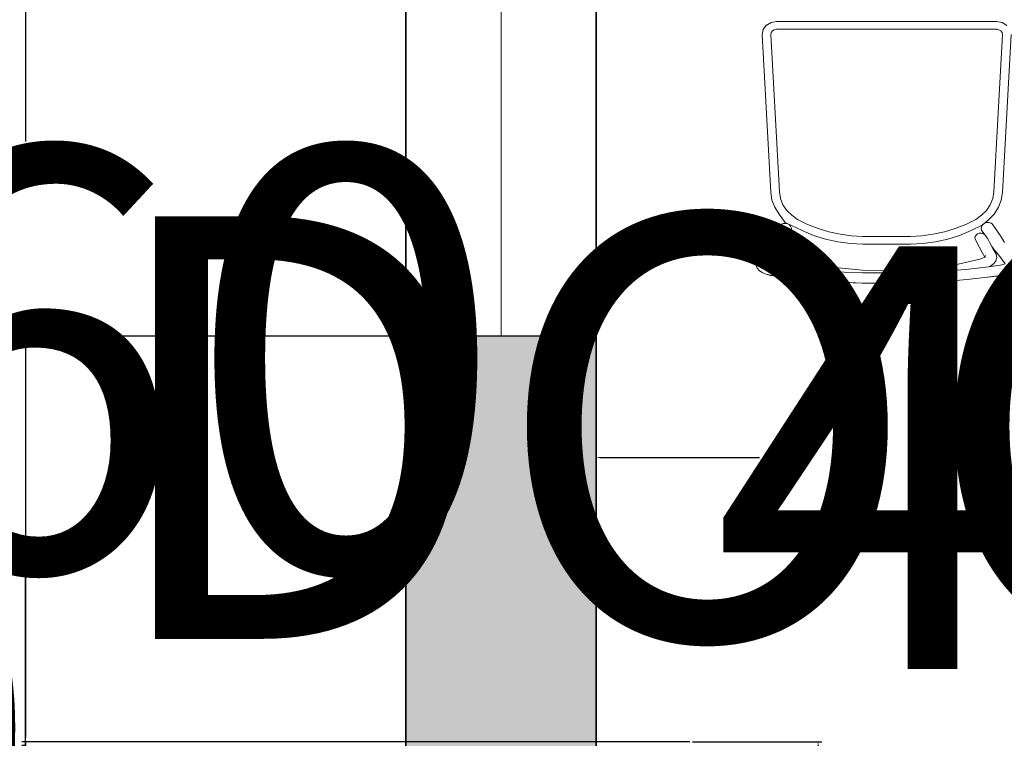
# Model space of a CAD drawing. Units: inches. Extents: x 305 to 776, y 38 to 479.
# Tile 5 of 14: x 372 to 419, y 231 to 265. Entities that reach past the tile are written whole.
import ezdxf

# ---------------------------------------------------------------- set-up
doc = ezdxf.new("R2010")
doc.units = ezdxf.units.IN
doc.header["$MEASUREMENT"] = 0
for name, color, linetype, lineweight in [('A-ANNO-DIMS', 2, 'Continuous', 18), ('A-FURN', 8, 'Continuous', 18), ('A-GLAZ', 4, 'Continuous', 20), ('A-WALL', 7, 'Continuous', 35), ('A-WALL-PATT', 252, 'Continuous', 13)]:
    doc.layers.add(name, color=color, linetype=linetype, lineweight=lineweight)
doc.styles.get("Standard").update_dxf_attribs({"font": 'arial.ttf'})
doc.dimstyles.get("Standard").update_dxf_attribs({"dimtxt": 20, "dimasz": 0.18, "dimexe": 0.18, "dimexo": 0.0625, "dimgap": 0.09, "dimtad": 0, "dimtih": 1, "dimtoh": 1, "dimdec": 4, "dimzin": 0, "dimdsep": 46, "dimtxsty": 'Standard', "dimcen": 0.09, "dimadec": 0, "dimazin": 0, "dimtfac": 1, "dimtdec": 4, "dimtofl": 0, "dimtmove": 0, "dimatfit": 3, "dimfxl": 1, "dimtolj": 1, "dimtzin": 0, "dimarcsym": 0})

# ---------------------------------------------------------------- blocks, each defined once
blk = doc.blocks.new('W3')
blk.add_line((906.212, 308.312), (886.612, 308.312))
blk.add_lwpolyline([(886.612, 303.812), (906.212, 303.812), (906.212, 312.812), (886.612, 312.812)])
blk = doc.blocks.new('D')
for p, q in [((1074.026, 474.114), (1073.821, 473.841)), ((1074.026, 474.113), (1073.821, 473.84)), ((1074.333, 474.296), (1074.026, 474.114)), ((1074.333, 474.295), (1074.026, 474.113)), ((1074.695, 474.36), (1074.333, 474.296)), ((1074.695, 474.359), (1074.333, 474.295)), ((1089.074, 474.36), (1074.695, 474.36)), ((1089.074, 474.359), (1074.695, 474.359)), ((1089.436, 474.296), (1089.074, 474.36)), ((1089.436, 474.295), (1089.074, 474.359)), ((1089.743, 474.114), (1089.436, 474.296)), ((1089.743, 474.113), (1089.436, 474.295)), ((1073.821, 473.841), (1073.749, 473.519)), ((1073.821, 473.84), (1073.749, 473.518)), ((1073.749, 473.519), (1074.316, 463.208)), ((1073.749, 473.518), (1074.316, 463.207)), ((1074.316, 473.518), (1074.345, 473.647)), ((1074.883, 463.232), (1074.316, 473.518)), ((1074.345, 473.647), (1074.427, 473.756)), ((1074.427, 473.756), (1074.55, 473.829)), ((1074.55, 473.829), (1074.695, 473.855)), ((1074.695, 473.855), (1089.074, 473.855)), ((1089.453, 473.518), (1088.886, 463.232)), ((1089.074, 473.855), (1089.219, 473.829)), ((1089.219, 473.829), (1089.342, 473.756)), ((1089.342, 473.756), (1089.424, 473.647)), ((1089.424, 473.647), (1089.453, 473.518)), ((1089.453, 463.208), (1090.02, 473.519)), ((1089.453, 463.207), (1090.02, 473.518)), ((1074.316, 463.208), (1074.397, 462.709)), ((1074.316, 463.207), (1074.397, 462.708)), ((1074.954, 462.807), (1074.883, 463.232)), ((1088.886, 463.232), (1088.815, 462.807)), ((1089.372, 462.709), (1089.453, 463.208)), ((1089.372, 462.708), (1089.453, 463.207)), ((1074.397, 462.709), (1074.58, 462.232)), ((1074.397, 462.708), (1074.58, 462.231)), ((1075.116, 462.403), (1074.954, 462.807)), ((1075.363, 462.034), (1075.116, 462.403)), ((1088.653, 462.403), (1088.406, 462.034)), ((1088.815, 462.807), (1088.653, 462.403)), ((1089.189, 462.232), (1089.372, 462.709)), ((1089.189, 462.231), (1089.372, 462.708)), ((1074.58, 462.232), (1074.859, 461.794)), ((1074.58, 462.231), (1074.859, 461.793)), ((1074.859, 461.794), (1075.262, 461.238)), ((1074.859, 461.793), (1075.262, 461.238)), ((1075.686, 461.714), (1075.363, 462.034)), ((1076.065, 461.447), (1075.686, 461.714)), ((1088.083, 461.714), (1087.704, 461.447)), ((1088.406, 462.034), (1088.083, 461.714)), ((1088.545, 461.409), (1088.91, 461.794)), ((1088.545, 461.408), (1088.91, 461.793)), ((1088.91, 461.794), (1089.189, 462.232)), ((1088.91, 461.793), (1089.189, 462.231)), ((1074.941, 461.071), (1074.459, 460.363)), ((1074.941, 461.071), (1074.459, 460.363)), ((1075.068, 461.151), (1074.941, 461.071)), ((1074.994, 461.113), (1074.941, 461.071)), ((1075.053, 461.145), (1074.994, 461.113)), ((1075.118, 461.169), (1075.053, 461.145)), ((1075.22, 461.186), (1075.068, 461.151)), ((1075.186, 461.183), (1075.118, 461.169)), ((1075.256, 461.187), (1075.186, 461.183)), ((1075.375, 461.17), (1075.22, 461.186)), ((1075.326, 461.181), (1075.256, 461.187)), ((1075.262, 461.238), (1075.339, 461.202)), ((1076.372, 460.712), (1075.262, 461.238)), ((1075.339, 461.202), (1075.326, 461.181)), ((1075.513, 461.105), (1075.375, 461.17)), ((1075.616, 461.001), (1075.513, 461.105)), ((1075.67, 460.87), (1075.616, 461.001)), ((1076.72, 461.12), (1076.065, 461.447)), ((1077.406, 460.848), (1076.72, 461.12)), ((1087.049, 461.12), (1086.363, 460.848)), ((1087.704, 461.447), (1087.049, 461.12)), ((1087.397, 460.712), (1088.111, 461.071)), ((1088.098, 461.017), (1088.06, 460.879)), ((1088.189, 461.132), (1088.098, 461.017)), ((1088.111, 461.071), (1088.545, 461.408)), ((1088.321, 461.212), (1088.189, 461.132)), ((1088.475, 461.243), (1088.321, 461.212)), ((1088.362, 461.267), (1088.545, 461.409)), ((1088.392, 461.234), (1088.362, 461.267)), ((1088.472, 461.244), (1088.392, 461.234)), ((1088.552, 461.241), (1088.472, 461.244)), ((1088.633, 461.224), (1088.475, 461.243)), ((1088.631, 461.225), (1088.552, 461.241)), ((1088.705, 461.196), (1088.631, 461.225)), ((1088.772, 461.155), (1088.633, 461.224)), ((1088.772, 461.156), (1088.705, 461.196)), ((1089.31, 460.363), (1088.772, 461.156)), ((1088.772, 461.155), (1089.31, 460.363)), ((1074.459, 460.363), (1074.192, 459.938)), ((1074.459, 460.363), (1074.192, 459.937)), ((1075.308, 460.2), (1075.415, 460.372)), ((1075.489, 460.462), (1075.415, 460.372)), ((1075.448, 460.42), (1075.61, 460.603)), ((1075.593, 460.525), (1075.489, 460.462)), ((1075.714, 460.554), (1075.593, 460.525)), ((1075.61, 460.603), (1075.668, 460.732)), ((1075.668, 460.732), (1075.67, 460.87)), ((1075.839, 460.545), (1075.714, 460.554)), ((1075.954, 460.5), (1075.839, 460.545)), ((1076.045, 460.423), (1075.954, 460.5)), ((1076.102, 460.324), (1076.045, 460.423)), ((1076.372, 460.712), (1077.118, 460.398)), ((1077.118, 460.398), (1077.895, 460.15)), ((1078.116, 460.631), (1077.406, 460.848)), ((1078.845, 460.472), (1078.116, 460.631)), ((1079.588, 460.372), (1078.845, 460.472)), ((1080.337, 460.332), (1079.588, 460.372)), ((1084.181, 460.372), (1083.432, 460.332)), ((1084.924, 460.472), (1084.181, 460.372)), ((1085.653, 460.631), (1084.924, 460.472)), ((1086.363, 460.848), (1085.653, 460.631)), ((1085.874, 460.15), (1086.651, 460.398)), ((1086.651, 460.398), (1087.397, 460.712)), ((1087.724, 460.423), (1087.667, 460.324)), ((1087.815, 460.5), (1087.724, 460.423)), ((1087.93, 460.545), (1087.815, 460.5)), ((1088.055, 460.554), (1087.93, 460.545)), ((1088.176, 460.525), (1088.055, 460.554)), ((1088.06, 460.879), (1088.08, 460.739)), ((1088.08, 460.739), (1088.155, 460.615)), ((1088.321, 460.42), (1088.155, 460.615)), ((1088.28, 460.462), (1088.176, 460.525)), ((1088.354, 460.372), (1088.28, 460.462)), ((1088.461, 460.2), (1088.354, 460.372)), ((1089.577, 459.938), (1089.31, 460.363)), ((1089.31, 460.363), (1089.577, 459.937)), ((1074.192, 459.938), (1073.839, 459.39)), ((1074.192, 459.937), (1073.839, 459.39)), ((1075.147, 459.905), (1074.97, 459.586)), ((1075.288, 460.169), (1075.147, 459.905)), ((1075.308, 460.2), (1075.288, 460.169)), ((1075.976, 459.888), (1075.827, 459.611)), ((1076.119, 460.213), (1075.976, 459.888)), ((1076.119, 460.213), (1076.102, 460.324)), ((1077.895, 460.15), (1078.696, 459.971)), ((1078.696, 459.971), (1079.513, 459.863)), ((1079.513, 459.863), (1080.337, 459.827)), ((1083.432, 460.332), (1080.337, 460.332)), ((1080.337, 459.827), (1083.432, 459.827)), ((1083.432, 459.827), (1084.256, 459.863)), ((1084.256, 459.863), (1085.073, 459.971)), ((1085.073, 459.971), (1085.874, 460.15)), ((1087.667, 460.324), (1087.65, 460.213)), ((1087.65, 460.213), (1087.793, 459.888)), ((1087.793, 459.888), (1087.942, 459.611)), ((1088.461, 460.2), (1088.481, 460.169)), ((1088.481, 460.169), (1088.622, 459.905)), ((1088.622, 459.905), (1088.799, 459.586)), ((1073.839, 459.39), (1073.441, 458.781)), ((1073.839, 459.39), (1073.441, 458.78)), ((1074.899, 459.526), (1074.503, 459.012)), ((1074.735, 459.167), (1074.693, 458.942)), ((1074.97, 459.586), (1074.735, 459.167)), ((1075.019, 459.675), (1074.899, 459.526)), ((1075.419, 459.083), (1075.441, 459.015)), ((1075.646, 459.285), (1075.472, 458.985)), ((1075.827, 459.611), (1075.646, 459.285)), ((1087.942, 459.611), (1088.123, 459.285)), ((1088.123, 459.285), (1088.297, 458.985)), ((1088.35, 459.083), (1088.328, 459.015)), ((1088.75, 459.675), (1088.87, 459.526)), ((1088.799, 459.586), (1089.034, 459.167)), ((1088.87, 459.526), (1089.265, 459.012)), ((1089.034, 459.167), (1089.076, 458.942)), ((1073.369, 458.627), (1073.341, 458.506)), ((1073.341, 458.506), (1073.369, 458.626)), ((1073.341, 458.506), (1073.38, 458.366)), ((1073.341, 458.506), (1073.38, 458.365)), ((1073.402, 458.733), (1073.369, 458.627)), ((1073.402, 458.732), (1073.369, 458.626)), ((1073.441, 458.781), (1073.402, 458.733)), ((1073.402, 458.732), (1073.441, 458.78)), ((1073.99, 458.675), (1074.082, 458.587)), ((1074.082, 458.587), (1074.149, 458.547)), ((1074.149, 458.547), (1074.284, 458.496)), ((1074.503, 459.012), (1074.155, 458.545)), ((1074.284, 458.496), (1074.454, 458.449)), ((1074.454, 458.449), (1075.569, 458.308)), ((1074.727, 458.826), (1074.693, 458.942)), ((1074.727, 458.826), (1074.764, 458.711)), ((1074.764, 458.711), (1074.907, 458.531)), ((1074.907, 458.531), (1075.103, 458.387)), ((1075.441, 459.015), (1075.456, 458.996)), ((1075.456, 458.996), (1075.511, 458.956)), ((1075.511, 458.956), (1075.628, 458.905)), ((1075.628, 458.905), (1075.79, 458.847)), ((1075.79, 458.847), (1077.219, 458.522)), ((1077.219, 458.522), (1078.734, 458.273)), ((1086.55, 458.522), (1085.035, 458.273)), ((1087.979, 458.847), (1086.55, 458.522)), ((1088.141, 458.905), (1087.979, 458.847)), ((1088.258, 458.956), (1088.141, 458.905)), ((1089.315, 458.449), (1088.2, 458.308)), ((1088.313, 458.996), (1088.258, 458.956)), ((1088.328, 459.015), (1088.313, 458.996)), ((1088.862, 458.531), (1088.666, 458.387)), ((1089.005, 458.711), (1088.862, 458.531)), ((1089.042, 458.826), (1089.005, 458.711)), ((1089.042, 458.826), (1089.076, 458.942)), ((1089.265, 459.012), (1089.614, 458.545)), ((1089.485, 458.496), (1089.315, 458.449)), ((1089.62, 458.547), (1089.485, 458.496)), ((1073.38, 458.366), (1073.421, 458.251)), ((1073.421, 458.25), (1073.38, 458.365)), ((1073.421, 458.251), (1073.589, 458.075)), ((1073.421, 458.25), (1073.589, 458.074)), ((1073.589, 458.075), (1073.794, 457.953)), ((1073.589, 458.074), (1073.794, 457.952)), ((1073.794, 457.953), (1074.023, 457.865)), ((1073.794, 457.952), (1074.023, 457.864)), ((1074.023, 457.865), (1074.289, 457.791)), ((1074.023, 457.864), (1074.289, 457.79)), ((1074.289, 457.791), (1075.47, 457.642)), ((1074.289, 457.79), (1075.47, 457.641)), ((1075.103, 458.387), (1075.165, 458.359)), ((1075.569, 458.308), (1076.732, 458.181)), ((1076.732, 458.181), (1077.91, 458.079)), ((1077.91, 458.079), (1079.101, 458.005)), ((1078.734, 458.273), (1080.296, 458.126)), ((1079.101, 458.005), (1080.302, 457.96)), ((1080.296, 458.126), (1081.884, 458.091)), ((1080.302, 457.96), (1081.509, 457.945)), ((1082.26, 457.945), (1081.509, 457.945)), ((1083.473, 458.126), (1081.884, 458.091)), ((1083.467, 457.96), (1082.26, 457.945)), ((1084.668, 458.005), (1083.467, 457.96)), ((1085.035, 458.273), (1083.473, 458.126)), ((1085.859, 458.079), (1084.668, 458.005)), ((1087.037, 458.181), (1085.859, 458.079)), ((1088.2, 458.308), (1087.037, 458.181)), ((1088.299, 457.642), (1089.48, 457.791)), ((1089.48, 457.79), (1088.299, 457.641)), ((1088.666, 458.387), (1088.604, 458.359)), ((1089.48, 457.791), (1089.746, 457.865)), ((1089.746, 457.864), (1089.48, 457.79)), ((1075.47, 457.642), (1076.649, 457.513)), ((1075.47, 457.641), (1076.649, 457.512)), ((1076.649, 457.513), (1077.847, 457.409)), ((1076.649, 457.512), (1077.847, 457.409)), ((1077.847, 457.409), (1079.059, 457.334)), ((1077.847, 457.409), (1079.059, 457.333)), ((1079.059, 457.334), (1080.28, 457.288)), ((1079.059, 457.333), (1080.28, 457.287)), ((1080.28, 457.288), (1081.503, 457.273)), ((1080.28, 457.287), (1081.503, 457.272)), ((1081.503, 457.273), (1082.266, 457.273)), ((1082.266, 457.272), (1081.503, 457.272)), ((1082.266, 457.273), (1083.489, 457.288)), ((1083.489, 457.287), (1082.266, 457.272)), ((1083.489, 457.288), (1084.71, 457.334)), ((1084.71, 457.333), (1083.489, 457.287)), ((1084.71, 457.334), (1085.922, 457.409)), ((1085.922, 457.409), (1084.71, 457.333)), ((1085.922, 457.409), (1087.12, 457.513)), ((1087.12, 457.512), (1085.922, 457.409)), ((1087.12, 457.513), (1088.299, 457.642)), ((1088.299, 457.641), (1087.12, 457.512))]:
    blk.add_line(p, q)
blk = doc.blocks.new('*D19')
at = {"layer": 'A-ANNO-DIMS', "color": 0, "lineweight": -2, "transparency": 16777216}
for p, q in [((557.633, 250.82), (557.633, 245.977)), ((589.133, 250.82), (589.133, 245.977)), ((557.633, 246.157), (557.453, 246.157)), ((588.953, 246.157), (557.813, 246.157))]:
    blk.add_line(p, q, dxfattribs=at)
at = {"layer": 'A-ANNO-DIMS', "color": 0, "transparency": 16777216}
for points in [[(557.813, 246.187), (557.813, 246.127), (557.633, 246.157)], [(588.953, 246.187), (588.953, 246.127), (589.133, 246.157)]]:
    blk.add_solid(points, dxfattribs=at)
at = {"layer": 'Defpoints', "color": 0, "transparency": 16777216}
for p in [(557.633, 250.882), (589.133, 250.882), (557.633, 246.157)]:
    blk.add_point(p, dxfattribs=at)
at = {"layer": 'A-ANNO-DIMS', "color": 0, "transparency": 16777216, "insert": (463.393, 246.157), "char_height": 20, "attachment_point": 5}
blk.add_mtext('\\A1;DOOR 32 TYP.', dxfattribs=at)
blk = doc.blocks.new('*D33')
at = {"layer": 'A-ANNO-DIMS', "color": 0, "lineweight": -2, "transparency": 16777216}
for p, q in [((440.927, 307.949), (449.29, 307.949)), ((449.11, 307.769), (449.11, 290.896)), ((449.11, 253.161), (449.11, 270.034)), ((440.927, 252.981), (449.29, 252.981))]:
    blk.add_line(p, q, dxfattribs=at)
at = {"layer": 'A-ANNO-DIMS', "color": 0, "transparency": 16777216}
for points in [[(449.08, 307.769), (449.14, 307.769), (449.11, 307.949)], [(449.08, 253.161), (449.14, 253.161), (449.11, 252.981)]]:
    blk.add_solid(points, dxfattribs=at)
at = {"layer": 'Defpoints', "color": 0, "transparency": 16777216}
for p in [(440.864, 307.949), (449.11, 307.949), (440.864, 252.981)]:
    blk.add_point(p, dxfattribs=at)
at = {"layer": 'A-ANNO-DIMS', "color": 0, "transparency": 16777216, "insert": (449.11, 280.465), "char_height": 20, "attachment_point": 5}
blk.add_mtext('\\A1;DINING SET 55', dxfattribs=at)
blk = doc.blocks.new('*D34')
at = {"layer": 'A-ANNO-DIMS', "color": 0, "lineweight": -2, "transparency": 16777216}
for p, q in [((399.621, 252.919), (399.621, 244.556)), ((440.864, 252.919), (440.864, 244.556)), ((399.801, 244.736), (407.356, 244.736)), ((440.684, 244.736), (433.129, 244.736))]:
    blk.add_line(p, q, dxfattribs=at)
at = {"layer": 'A-ANNO-DIMS', "color": 0, "transparency": 16777216}
for points in [[(399.801, 244.766), (399.801, 244.706), (399.621, 244.736)], [(440.684, 244.766), (440.684, 244.706), (440.864, 244.736)]]:
    blk.add_solid(points, dxfattribs=at)
at = {"layer": 'Defpoints', "color": 0, "transparency": 16777216}
for p in [(399.621, 252.981), (440.864, 252.981), (440.864, 244.736)]:
    blk.add_point(p, dxfattribs=at)
at = {"layer": 'A-ANNO-DIMS', "color": 0, "transparency": 16777216, "insert": (420.242, 244.736), "char_height": 20, "attachment_point": 5}
blk.add_mtext('\\A1;41', dxfattribs=at)
blk = doc.blocks.new('*D37')
at = {"layer": 'A-ANNO-DIMS', "color": 0, "lineweight": -2, "transparency": 16777216}
for p, q in [((476.346, 237.029), (483.222, 237.029)), ((483.042, 236.849), (483.042, 224.939)), ((483.042, 192.153), (483.042, 204.063)), ((476.346, 191.973), (483.222, 191.973))]:
    blk.add_line(p, q, dxfattribs=at)
at = {"layer": 'A-ANNO-DIMS', "color": 0, "transparency": 16777216}
for points in [[(483.012, 236.849), (483.072, 236.849), (483.042, 237.029)], [(483.012, 192.153), (483.072, 192.153), (483.042, 191.973)]]:
    blk.add_solid(points, dxfattribs=at)
at = {"layer": 'Defpoints', "color": 0, "transparency": 16777216}
for p in [(476.283, 237.029), (483.042, 237.029), (476.283, 191.973)]:
    blk.add_point(p, dxfattribs=at)
at = {"layer": 'A-ANNO-DIMS', "color": 0, "transparency": 16777216, "insert": (483.042, 214.501), "char_height": 20, "attachment_point": 5}
blk.add_mtext('\\A1;COFFEE TABLE 45', dxfattribs=at)
blk = doc.blocks.new('*D39')
at = {"layer": 'A-ANNO-DIMS', "color": 0, "lineweight": -2, "transparency": 16777216}
for p, q in [((404.195, 231.292), (410.313, 231.292)), ((410.133, 231.112), (410.133, 221.593)), ((410.133, 191.472), (410.133, 200.99)), ((404.195, 191.292), (410.313, 191.292))]:
    blk.add_line(p, q, dxfattribs=at)
at = {"layer": 'A-ANNO-DIMS', "color": 0, "transparency": 16777216}
for points in [[(410.103, 231.112), (410.163, 231.112), (410.133, 231.292)], [(410.103, 191.472), (410.163, 191.472), (410.133, 191.292)]]:
    blk.add_solid(points, dxfattribs=at)
at = {"layer": 'Defpoints', "color": 0, "transparency": 16777216}
for p in [(404.133, 231.292), (410.133, 231.292), (404.133, 191.292)]:
    blk.add_point(p, dxfattribs=at)
at = {"layer": 'A-ANNO-DIMS', "color": 0, "transparency": 16777216, "insert": (410.133, 211.292), "char_height": 20, "attachment_point": 5}
blk.add_mtext('\\A1;TV 40', dxfattribs=at)
blk = doc.blocks.new('*D46')
at = {"layer": 'A-ANNO-DIMS', "color": 0, "lineweight": -2, "transparency": 16777216}
for p, q in [((390.57, 429.382), (372.451, 429.382)), ((372.631, 429.202), (372.631, 259.69)), ((372.631, 69.562), (372.631, 239.074)), ((390.57, 69.382), (372.451, 69.382))]:
    blk.add_line(p, q, dxfattribs=at)
at = {"layer": 'A-ANNO-DIMS', "color": 0, "transparency": 16777216}
for points in [[(372.601, 429.202), (372.661, 429.202), (372.631, 429.382)], [(372.601, 69.562), (372.661, 69.562), (372.631, 69.382)]]:
    blk.add_solid(points, dxfattribs=at)
at = {"layer": 'Defpoints', "color": 0, "transparency": 16777216}
for p in [(372.631, 429.382), (390.633, 429.382), (390.633, 69.382)]:
    blk.add_point(p, dxfattribs=at)
at = {"layer": 'A-ANNO-DIMS', "color": 0, "transparency": 16777216, "insert": (372.631, 249.382), "char_height": 20, "attachment_point": 5}
blk.add_mtext('\\A1;360', dxfattribs=at)
blk = doc.blocks.new('*D62')
at = {"layer": 'A-ANNO-DIMS', "color": 0, "lineweight": -2, "transparency": 16777216}
for p, q in [((399.633, 336.32), (399.633, 51.201)), ((423.233, 336.32), (423.233, 51.201)), ((399.813, 51.381), (423.053, 51.381)), ((423.233, 51.381), (423.413, 51.381))]:
    blk.add_line(p, q, dxfattribs=at)
at = {"layer": 'A-ANNO-DIMS', "color": 0, "transparency": 16777216}
for points in [[(399.813, 51.411), (399.813, 51.351), (399.633, 51.381)], [(423.053, 51.411), (423.053, 51.351), (423.233, 51.381)]]:
    blk.add_solid(points, dxfattribs=at)
at = {"layer": 'Defpoints', "color": 0, "transparency": 16777216}
for p in [(399.633, 336.382), (423.233, 336.382), (423.233, 51.381)]:
    blk.add_point(p, dxfattribs=at)
at = {"layer": 'A-ANNO-DIMS', "color": 0, "transparency": 16777216, "insert": (449.642, 51.381), "char_height": 20, "attachment_point": 5}
blk.add_mtext('\\A1;23.6', dxfattribs=at)
blk = doc.blocks.new('*D65')
at = {"layer": 'A-ANNO-DIMS', "color": 0, "lineweight": -2, "transparency": 16777216}
for p, q in [((399.633, 351.219), (399.633, 51.201)), ((421.89, 351.219), (421.89, 51.201)), ((399.813, 51.381), (421.71, 51.381)), ((421.89, 51.381), (422.07, 51.381))]:
    blk.add_line(p, q, dxfattribs=at)
at = {"layer": 'A-ANNO-DIMS', "color": 0, "transparency": 16777216}
for points in [[(399.813, 51.411), (399.813, 51.351), (399.633, 51.381)], [(421.71, 51.411), (421.71, 51.351), (421.89, 51.381)]]:
    blk.add_solid(points, dxfattribs=at)
at = {"layer": 'Defpoints', "color": 0, "transparency": 16777216}
for p in [(399.633, 351.281), (421.89, 351.281), (421.89, 51.381)]:
    blk.add_point(p, dxfattribs=at)
at = {"layer": 'A-ANNO-DIMS', "color": 0, "transparency": 16777216, "insert": (463.844, 51.381), "char_height": 20, "attachment_point": 5}
blk.add_mtext('\\A1;22.257', dxfattribs=at)
blk = doc.blocks.new('*D74')
at = {"layer": 'A-ANNO-DIMS', "color": 0, "lineweight": -2, "transparency": 16777216}
for p, q in [((399.57, 250.482), (372.451, 250.482)), ((372.631, 250.302), (372.631, 231.472)), ((404.07, 231.292), (372.451, 231.292)), ((372.631, 231.112), (372.451, 231.112)), ((372.631, 231.292), (372.631, 231.112))]:
    blk.add_line(p, q, dxfattribs=at)
at = {"layer": 'A-ANNO-DIMS', "color": 0, "transparency": 16777216}
for points in [[(372.601, 250.302), (372.661, 250.302), (372.631, 250.482)], [(372.601, 231.472), (372.661, 231.472), (372.631, 231.292)]]:
    blk.add_solid(points, dxfattribs=at)
at = {"layer": 'Defpoints', "color": 0, "transparency": 16777216}
for p in [(399.633, 250.482), (372.631, 231.292), (404.133, 231.292)]:
    blk.add_point(p, dxfattribs=at)
at = {"layer": 'A-ANNO-DIMS', "color": 0, "transparency": 16777216, "insert": (339.537, 231.112), "char_height": 20, "attachment_point": 5}
blk.add_mtext('\\A1;19.19', dxfattribs=at)

msp = doc.modelspace()

# ---------------------------------------------------------------- hatches: boundary and pattern name
at = {"layer": 'A-WALL-PATT'}
h = msp.add_hatch(color=256, dxfattribs=at)
h.dxf.hatch_style = 1
h.paths.add_polyline_path([(481.3329, 429.382), (390.6329, 429.382), (390.6329, 398.067), (399.6329, 398.067), (399.6329, 420.382), (465.6329, 420.382), (465.6329, 331.882), (470.1329, 331.882), (470.1329, 355.882), (512.1329, 355.882), (512.1329, 337.282), (512.1329, 337.282), (515.8592, 337.282), (516.6329, 337.282), (516.6329, 360.382), (513.3171, 360.382), (470.1329, 360.382), (470.1329, 420.382), (481.3329, 420.382)])
h.paths.add_polyline_path([(630.6329, 429.382), (500.9329, 429.382), (500.9329, 420.382), (502.8693, 420.382), (512.1329, 420.382), (512.1329, 391.882), (516.6329, 391.882), (516.6329, 420.382), (621.6329, 420.382), (621.6329, 388.182), (630.6329, 388.182)])
h.paths.add_polyline_path([(630.6329, 329.382), (621.6329, 329.382), (621.6329, 301.882), (512.1329, 301.882), (512.1329, 297.382), (515.8592, 297.382), (557.6329, 297.382), (621.6329, 297.382), (621.6329, 286.182), (630.6329, 286.182)])
h.paths.add_polyline_path([(630.6329, 266.582), (621.6329, 266.582), (621.6329, 255.382), (589.1329, 255.382), (589.1329, 250.882), (621.6329, 250.882), (621.6329, 226.282), (630.6329, 226.282)])
h.paths.add_polyline_path([(630.6329, 167.482), (621.6329, 167.482), (621.6329, 149.1444), (621.6329, 142.882), (516.6329, 142.882), (516.6329, 261.982), (512.1329, 261.982), (512.1329, 138.382), (621.6329, 138.382), (621.6329, 78.382), (512.1329, 78.382), (512.1329, 69.382), (630.6329, 69.382)])
h.paths.add_polyline_path([(464.1329, 138.382), (476.7329, 138.382), (476.7329, 142.1084), (476.7329, 142.882), (459.6329, 142.882), (459.6329, 78.382), (399.6329, 78.382), (399.6329, 98.582), (390.6329, 98.582), (390.6329, 69.382), (464.1329, 69.382)])
h.paths.add_polyline_path([(459.6329, 142.882), (439.3329, 142.882), (439.3329, 138.382), (459.6329, 138.382)], flags=17)
h.paths.add_polyline_path([(399.6329, 138.382), (403.9329, 138.382), (403.9329, 141.5545), (403.9329, 141.5545), (403.9329, 142.882), (399.6329, 142.882), (399.6329, 250.4819), (390.6329, 250.4819), (390.6329, 118.182), (399.6329, 118.182)])
h.paths.add_polyline_path([(399.6329, 331.882), (428.2629, 331.882), (428.2629, 336.382), (399.6329, 336.382), (399.6329, 358.697), (390.6329, 358.697), (390.6329, 309.2819), (399.6329, 309.2819)])

# ---------------------------------------------------------------- linework, layer by layer
at = {"layer": 'A-WALL'}
msp.add_line((399.6329, 331.882), (399.6329, 142.882), dxfattribs=at)
msp.add_lwpolyline([(390.6329, 69.382), (630.6329, 69.382), (630.6329, 429.382), (390.6329, 429.382)], close=True, dxfattribs=at)

# ---------------------------------------------------------------- block references
at = {"layer": 'A-FURN', "xscale": 0.724692399516523, "yscale": 0.724692399516523, "zscale": 0.724692399516523}
msp.add_blockref('D', (-370.653, -78.4001), dxfattribs=at)
at = {"layer": 'A-GLAZ', "rotation": 270}
msp.add_blockref('W3', (86.8213, 1156.694), dxfattribs=at)

# ---------------------------------------------------------------- dimensions: what is measured, and where the dimension line sits
at = {"layer": 'A-ANNO-DIMS'}
for base, p1, p2, override, picture, middle in [((372.6314, 429.382), (390.6329, 69.382), (390.6329, 429.382), {"dimdec": 0, "dimlfac": 1, "dimrnd": 0, "dimzin": 0, "dimdsep": 46, "dimlunit": 2}, '*D46', (372.6314, 249.382)), ((372.6314, 231.2915), (399.6329, 250.4819), (404.1329, 231.2915), {"dimdec": 2, "dimlfac": 1, "dimrnd": 0, "dimzin": 0, "dimdsep": 46, "dimlunit": 2}, '*D74', (339.5374, 231.1115))]:
    dim = msp.add_linear_dim(base=base, p1=p1, p2=p2, angle=90, dimstyle='Standard', override=override, dxfattribs=at)
    dim.commit()
    dim.dimension.update_dxf_attribs({"geometry": picture, "text_midpoint": middle})
for base, p1, p2, override, picture, middle in [((421.8895, 51.3805), (399.6329, 351.2815), (421.8895, 351.2815), {"dimdec": 3, "dimlfac": 1, "dimrnd": 0, "dimzin": 0, "dimdsep": 46, "dimlunit": 2}, '*D65', (463.8444, 51.3805)), ((423.2329, 51.3805), (399.6329, 336.382), (423.2329, 336.382), {"dimdec": 1, "dimlfac": 1, "dimrnd": 0, "dimzin": 0, "dimdsep": 46, "dimlunit": 2}, '*D62', (449.6421, 51.3805)), ((440.8644, 244.7363), (399.6205, 252.9815), (440.8644, 252.9815), {"dimdec": 0, "dimlfac": 1, "dimrnd": 0, "dimzin": 0, "dimdsep": 46, "dimlunit": 2}, '*D34', (420.2425, 244.7363))]:
    dim = msp.add_linear_dim(base=base, p1=p1, p2=p2, dimstyle='Standard', override=override, dxfattribs=at)
    dim.commit()
    dim.dimension.update_dxf_attribs({"geometry": picture, "text_midpoint": middle})
for base, p1, p2, angle, text, picture, middle in [((449.1096, 307.9493), (440.8644, 252.9815), (440.8644, 307.9493), 90, 'DINING SET <>', '*D33', (449.1096, 280.4654)), ((557.6329062952, 246.15704135), (589.1329062952, 250.88204135), (557.6329062952, 250.88204135), 180, 'DOOR <> TYP.', '*D19', (463.3929199378, 246.15704135)), ((483.0416, 237.0288), (476.2832, 191.9726), (476.2832, 237.0288), 90, 'COFFEE TABLE <>', '*D37', (483.0416, 214.5007)), ((410.1329, 231.2915), (404.1329, 191.2915), (404.1329, 231.2915), 90, 'TV <>', '*D39', (410.1329, 211.2915))]:
    dim = msp.add_linear_dim(base=base, p1=p1, p2=p2, angle=angle, text=text, dimstyle='Standard', override={"dimdec": 0, "dimlfac": 1, "dimrnd": 0, "dimzin": 0, "dimdsep": 46, "dimlunit": 2}, dxfattribs=at)
    dim.commit()
    dim.dimension.update_dxf_attribs({"geometry": picture, "text_midpoint": middle})

doc.saveas('drawing.dxf')
